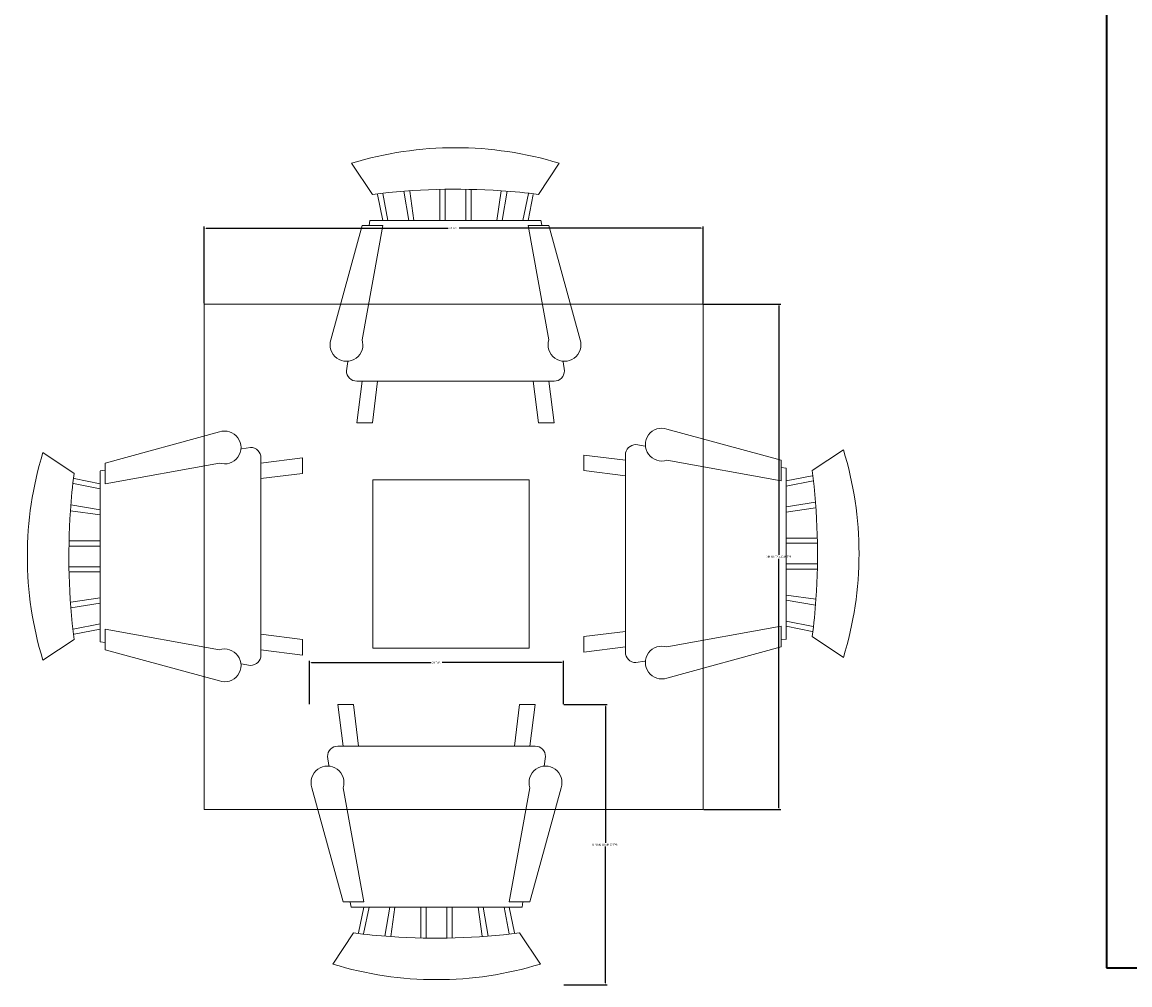
# Model space of a CAD drawing. Units: inches. Extents: x 108 to 613, y 1573 to 2319.
# Tile 9 of 11: x 327 to 434, y 2132 to 2225. Entities that reach past the tile are written whole.
import ezdxf

# ---------------------------------------------------------------- set-up
doc = ezdxf.new("R2010")
doc.units = ezdxf.units.IN
for name, color, linetype, lineweight in [('A-ANNO-DIMS', 2, 'Continuous', 18), ('furniture', 2, 'Continuous', 18), ('wall', 6, 'Continuous', 35)]:
    doc.layers.add(name, color=color, linetype=linetype, lineweight=lineweight)
doc.styles.get("Standard").update_dxf_attribs({"font": 'arial.ttf'})
doc.dimstyles.get("Standard").update_dxf_attribs({"dimtxt": 0.18, "dimasz": 0.18, "dimexe": 0.18, "dimexo": 0.0625, "dimgap": 0.09, "dimtad": 0, "dimtih": 1, "dimtoh": 1, "dimdec": 4, "dimzin": 0, "dimdsep": 46, "dimtxsty": 'Standard', "dimcen": 0.09, "dimadec": 0, "dimazin": 0, "dimtfac": 1, "dimtdec": 4, "dimtofl": 0, "dimtmove": 0, "dimatfit": 3, "dimfxl": 1, "dimtolj": 1, "dimtzin": 0, "dimarcsym": 0})

# ---------------------------------------------------------------- blocks, each defined once
blk = doc.blocks.new('Chair - Rocking')
for p, q in [((-8, -4.5), (-10, -1.5)), ((8, -4.5), (10, -1.5)), ((-4.5, -7), (-4.96674, -4.19951)), ((-4, -7), (-4.40532, -4.16272)), ((-1.5, -4.05012), (-1.5, -7)), ((-1, -7), (-1, -4.05012)), ((1, -7), (1, -4.04655)), ((1.5, -4.05012), (1.5, -7)), ((4, -7), (4.40187, -4.18694)), ((4.5, -7), (4.96761, -4.19437)), ((-7.5, -4.5), (-7, -7)), ((-6.5, -7), (-7.02225, -4.43)), ((6.5, -7), (7, -4.4057)), ((7.5, -4.5), (7, -7)), ((-8.23428, -6.99939), (-8.3093, -7.47958)), ((-8.23041, -7), (8.23915, -7)), ((8.31071, -7.48854), (8.23449, -7.00073)), ((-9, -7.5), (-12, -18.49999)), ((-7, -7.5), (-9, -7.5)), ((-9, -18.49999), (-7, -7.5)), ((7, -7.5), (9, -7.5)), ((9, -18.49999), (7, -7.5)), ((9, -7.5), (12, -18.49999)), ((-10.36644, -20.64523), (-10.5, -21.49999)), ((10.5, -21.49999), (10.3575, -20.58798)), ((-9, -22.49999), (-9.5, -26.49999)), ((0, -22.49999), (-9.5, -22.49999)), ((-8, -26.49999), (-7.5, -22.49999)), ((0, -22.49999), (9.5, -22.49999)), ((8, -26.49999), (7.5, -22.49999)), ((9, -22.49999), (9.5, -26.49999)), ((-9.5, -26.49999), (-8, -26.49999)), ((9.5, -26.49999), (8, -26.49999))]:
    blk.add_line(p, q)
for centre, radius, start, end in [((0, -34.08333), 34.08333, 72.93847, 107.0615), ((0, -68.25004), 64.25, 93.92211, 97.15267), ((0, -68.25004), 64.25, 82.84733, 93.92211), ((-10.5, -18.99999), 1.58114, 161.5651, 18.43495), ((10.5, -18.99999), 1.58114, 161.5651, 18.43495), ((-9.5, -21.49999), 1, 180, 270), ((9.5, -21.49999), 1, 270, 0)]:
    blk.add_arc(centre, radius, start, end)
blk = doc.blocks.new('DINING-TABLE')
for points in [[(0, 48.71), (48.06, 48.71), (48.06, 0), (0, 0)], [(16.26, 33.17), (31.3, 33.17), (31.3, 16.93), (16.26, 16.93)]]:
    blk.add_lwpolyline(points, close=True)
blk = doc.blocks.new('*D19')
at = {"layer": 'A-ANNO-DIMS', "color": 0, "lineweight": -2, "transparency": 16777216}
for p, q in [((379.02, 2159.48), (383.19, 2159.48)), ((383.01, 2159.3), (383.01, 2146.16)), ((383.01, 2132.66), (383.01, 2145.8)), ((379.02, 2132.48), (383.19, 2132.48))]:
    blk.add_line(p, q, dxfattribs=at)
at = {"layer": 'A-ANNO-DIMS', "color": 0, "transparency": 16777216}
for points in [[(382.98, 2159.3), (383.04, 2159.3), (383.01, 2159.48)], [(382.98, 2132.66), (383.04, 2132.66), (383.01, 2132.48)]]:
    blk.add_solid(points, dxfattribs=at)
at = {"layer": 'Defpoints', "color": 0, "transparency": 16777216}
for p in [(378.96, 2159.48), (378.96, 2132.48), (383.01, 2132.48)]:
    blk.add_point(p, dxfattribs=at)
at = {"layer": 'A-ANNO-DIMS', "color": 0, "transparency": 16777216, "insert": (383.01, 2145.98), "char_height": 0.18, "attachment_point": 5}
blk.add_mtext('\\A1;DINING CHAIR 27 TYP.', dxfattribs=at)
blk = doc.blocks.new('*D20')
at = {"layer": 'A-ANNO-DIMS', "color": 0, "lineweight": -2, "transparency": 16777216}
for p, q in [((354.52, 2159.54), (354.52, 2163.71)), ((354.7, 2163.53), (366.21, 2163.53)), ((378.78, 2163.53), (367.27, 2163.53)), ((378.96, 2159.54), (378.96, 2163.71))]:
    blk.add_line(p, q, dxfattribs=at)
at = {"layer": 'A-ANNO-DIMS', "color": 0, "transparency": 16777216}
for points in [[(354.7, 2163.56), (354.7, 2163.5), (354.52, 2163.53)], [(378.78, 2163.56), (378.78, 2163.5), (378.96, 2163.53)]]:
    blk.add_solid(points, dxfattribs=at)
at = {"layer": 'Defpoints', "color": 0, "transparency": 16777216}
for p in [(378.96, 2163.53), (354.52, 2159.48), (378.96, 2159.48)]:
    blk.add_point(p, dxfattribs=at)
at = {"layer": 'A-ANNO-DIMS', "color": 0, "transparency": 16777216, "insert": (366.74, 2163.53), "char_height": 0.18, "attachment_point": 5}
blk.add_mtext('\\A1;24 TYP.', dxfattribs=at)
blk = doc.blocks.new('*D37')
at = {"layer": 'A-ANNO-DIMS', "color": 0, "lineweight": -2, "transparency": 16777216}
for p, q in [((392.48, 2198.08), (399.91, 2198.08)), ((399.73, 2197.9), (399.73, 2173.91)), ((399.73, 2149.55), (399.73, 2173.54)), ((392.48, 2149.37), (399.91, 2149.37))]:
    blk.add_line(p, q, dxfattribs=at)
at = {"layer": 'A-ANNO-DIMS', "color": 0, "transparency": 16777216}
for points in [[(399.7, 2197.9), (399.76, 2197.9), (399.73, 2198.08)], [(399.7, 2149.55), (399.76, 2149.55), (399.73, 2149.37)]]:
    blk.add_solid(points, dxfattribs=at)
at = {"layer": 'Defpoints', "color": 0, "transparency": 16777216}
for p in [(392.42, 2198.08), (392.42, 2149.37), (399.73, 2149.37)]:
    blk.add_point(p, dxfattribs=at)
at = {"layer": 'A-ANNO-DIMS', "color": 0, "transparency": 16777216, "insert": (399.73, 2173.73), "char_height": 0.18, "attachment_point": 5}
blk.add_mtext('\\A1;DINING TABLE 49 TYP.', dxfattribs=at)
blk = doc.blocks.new('*D38')
at = {"layer": 'A-ANNO-DIMS', "color": 0, "lineweight": -2, "transparency": 16777216}
for p, q in [((344.36, 2198.14), (344.36, 2205.57)), ((392.42, 2198.14), (392.42, 2205.57)), ((344.54, 2205.39), (367.86, 2205.39)), ((392.24, 2205.39), (368.92, 2205.39))]:
    blk.add_line(p, q, dxfattribs=at)
at = {"layer": 'A-ANNO-DIMS', "color": 0, "transparency": 16777216}
for points in [[(344.54, 2205.42), (344.54, 2205.36), (344.36, 2205.39)], [(392.24, 2205.42), (392.24, 2205.36), (392.42, 2205.39)]]:
    blk.add_solid(points, dxfattribs=at)
at = {"layer": 'Defpoints', "color": 0, "transparency": 16777216}
for p in [(392.42, 2205.39), (344.36, 2198.08), (392.42, 2198.08)]:
    blk.add_point(p, dxfattribs=at)
at = {"layer": 'A-ANNO-DIMS', "color": 0, "transparency": 16777216, "insert": (368.39, 2205.39), "char_height": 0.18, "attachment_point": 5}
blk.add_mtext('\\A1;48 TYP.', dxfattribs=at)

msp = doc.modelspace()

# ---------------------------------------------------------------- linework, layer by layer
at = {"layer": 'wall'}
for p, q in [((431.2753, 2227.1125), (431.2753, 2134.1125)), ((431.2753, 2134.1125), (435.7753, 2134.1125))]:
    msp.add_line(p, q, dxfattribs=at)

# ---------------------------------------------------------------- block references
at = {"layer": 'furniture', "xscale": -1}
msp.add_blockref('Chair - Rocking', (368.5653, 2213.1483), dxfattribs=at)
at = {"layer": 'furniture', "extrusion": (0, 0, -1), "zscale": -1, "rotation": 180}
msp.add_blockref('DINING-TABLE', (-344.357, 2198.082), dxfattribs=at)
at = {"layer": 'furniture', "xscale": -1}
for p, rotation in [((407.4365, 2174.0358), 270), ((327.3278, 2173.7632), 90), ((366.7413, 2132.9793), 180)]:
    msp.add_blockref('Chair - Rocking', p, dxfattribs=dict(at, rotation=rotation))

# ---------------------------------------------------------------- dimensions: what is measured, and where the dimension line sits
at = {"layer": 'A-ANNO-DIMS'}
for base, p1, p2, picture, middle in [((392.4218, 2205.3884), (344.3572, 2198.0816), (392.4218, 2198.0816), '*D38', (368.3895, 2205.3884)), ((378.9588, 2163.5293), (354.5238, 2159.4793), (378.9588, 2159.4793), '*D20', (366.7413, 2163.5293))]:
    dim = msp.add_linear_dim(base=base, p1=p1, p2=p2, text='<> TYP.', dimstyle='Standard', override={"dimdec": 0, "dimlfac": 1, "dimrnd": 0, "dimzin": 0, "dimdsep": 46, "dimlunit": 2}, dxfattribs=at)
    dim.commit()
    dim.dimension.update_dxf_attribs({"geometry": picture, "text_midpoint": middle})
for base, p1, p2, text, picture, middle in [((399.7285, 2149.3702), (392.4218, 2198.0816), (392.4218, 2149.3702), 'DINING TABLE <> TYP.', '*D37', (399.7285, 2173.7259)), ((383.0088, 2132.4793), (378.9588, 2159.4793), (378.9588, 2132.4793), 'DINING CHAIR <> TYP.', '*D19', (383.0088, 2145.9793))]:
    dim = msp.add_linear_dim(base=base, p1=p1, p2=p2, angle=270, text=text, dimstyle='Standard', override={"dimdec": 0, "dimlfac": 1, "dimrnd": 0, "dimzin": 0, "dimdsep": 46, "dimlunit": 2}, dxfattribs=at)
    dim.commit()
    dim.dimension.update_dxf_attribs({"geometry": picture, "text_midpoint": middle})

doc.saveas('drawing.dxf')
